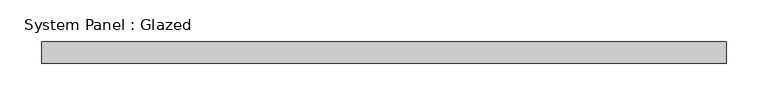
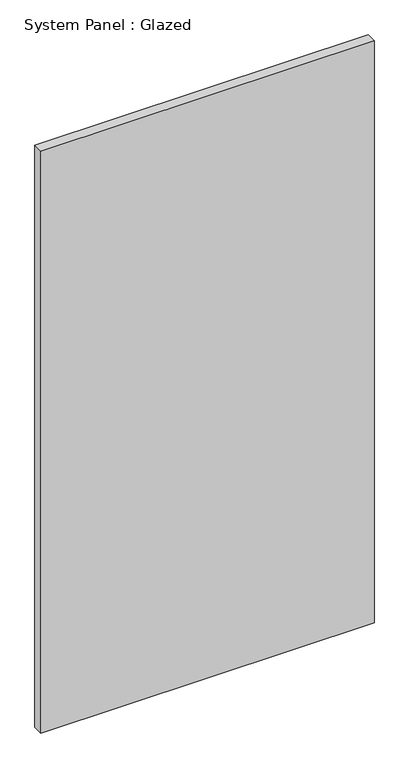
"""IFC4 building model written with IfcOpenShell, lengths in millimetres: plate geometry, System Panel : Glazed."""

from ifc_helpers import new_model, si_unit, origin, origin_with_axes, place, context, project, spatial, polyline, outline, extrude, source, transform, mapped, element, save


def system_panel_glazed_f34af49f(model_context):
    return source(origin(), model_context, "Body", "SweptSolid", [
        extrude(outline(polyline([(409.575, 19.05), (-409.575, 19.05), (-409.575, 44.45), (409.575, 44.45), (409.575, 19.05)])), origin_with_axes(), (0.0, 0.0, 1.0), 1512.8191133),
    ])


if __name__ == "__main__":
    model = new_model("IFC4")
    model_context = context("Model", 3, world=origin())
    ifc_project = project(units=[si_unit("LENGTHUNIT", "METRE", prefix="MILLI")], contexts=[model_context])
    site = spatial("IfcSite", under=ifc_project)
    building = spatial("IfcBuilding", under=site)
    placement = place(None, origin())
    system_panel_glazed_shape = system_panel_glazed_f34af49f(model_context)
    element("IfcPlate", 1, ObjectType="System Panel : Glazed", at=placement, inside=building, context=model_context, shape_type="MappedRepresentation", body=[
        mapped(system_panel_glazed_shape, transform((0.0, 0.0, 0.0), x_axis=(1.0, 0.0, 0.0), y_axis=(0.0, 1.0, 0.0), z_axis=(0.0, 0.0, 1.0))),
    ])
    save(model, "model.ifc")

# Revit data of these elements
# Type "System Panel : Glazed"
#   Construction Type Id = "GSP4R"
#   Analytic Construction = "1/8 in Pilkington single glazing"
#   Visual Light Transmittance = 0.9
#   Solar Heat Gain Coefficient = 0.86
#   Heat Transfer Coefficient (U) = 1.18115 BTU/(h·ft²·°F)
#   Define Thermal Properties by = 1
# Element 1 (IfcPlate, "System Panel : Glazed")
#   Materials on its faces: "Glass"
# Materials
#   "Glass": class "Glass", colour RGB 0 128 192, transparency 0.75, Description = "Soda Lime Glass", Cost = 0
